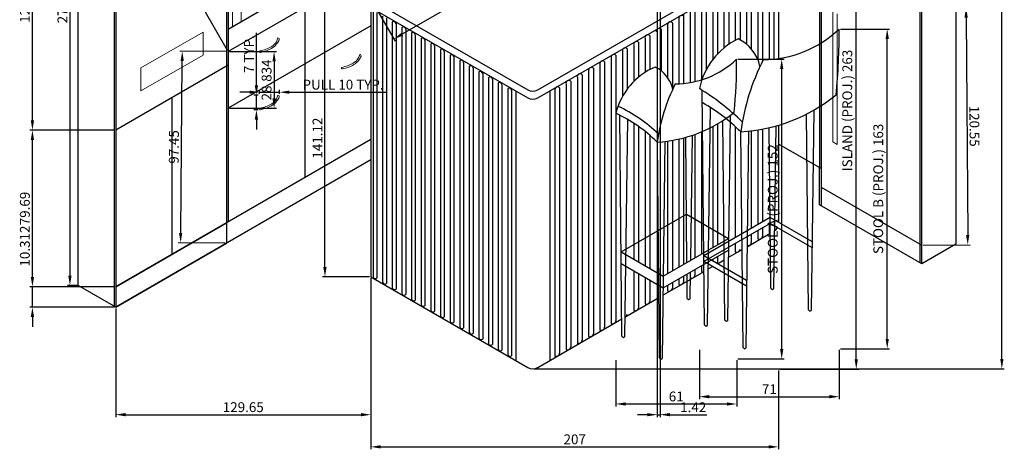
# Model space of a CAD drawing. Units: centimetres. Extents: x 2148 to 2649, y 4226 to 4785.
# Tile 1 of 6: x 2148 to 2649, y 4226 to 4445. Entities that reach past the tile are written whole.
import ezdxf

# ---------------------------------------------------------------- set-up
doc = ezdxf.new("R2010")
doc.units = ezdxf.units.CM
for name, color, linetype, lineweight in [('A-ANNO-DIMS', 63, 'Continuous', 18), ('A-ANNO-REFR', 8, 'Continuous', 13), ('A-EQPM', 30, 'Continuous', 18), ('A-FLOR-BSPL', 21, 'Continuous', 13), ('A-FLOR-CASE', 21, 'Continuous', 25), ('A-FLOR-CASE-HDW', 21, 'Continuous', 18), ('A-FLOR-CASE-TALL', 30, 'Continuous', 30), ('A-FLOR-CTOP', 21, 'Continuous', 25), ('CHAIR', 32, 'Continuous', 25), ('TABLE', 30, 'Continuous', 25)]:
    doc.layers.add(name, color=color, linetype=linetype, lineweight=lineweight)
doc.styles.get("Standard").update_dxf_attribs({"font": 'arial.ttf'})
doc.dimstyles.new('ISO-25', dxfattribs={"dimtxt": 5, "dimasz": 5, "dimexe": 1.25, "dimexo": 0.625, "dimtad": 1, "dimdec": 1, "dimtxsty": 'Standard', "dimcen": 2.5, "dimadec": 0, "dimazin": 0, "dimtfac": 1, "dimtdec": 1, "dimtmove": 0, "dimatfit": 3, "dimfxl": 1, "dimarcsym": 0})

# ---------------------------------------------------------------- blocks, each defined once
blk = doc.blocks.new('RECTANGLE')
for p, q in [((2256.66, 4502.65), (2260.99, 4505.15)), ((2260.99, 4443.76), (2260.99, 4505.15)), ((2256.66, 4502.65), (2256.66, 4441.26)), ((2256.66, 4441.26), (2260.99, 4443.76))]:
    blk.add_line(p, q)
blk = doc.blocks.new('*D4')
at = {"layer": 'A-ANNO-DIMS', "color": 0, "lineweight": -2, "transparency": 16777216}
for p, q in [((2177.63, 4587.69), (2172.75, 4587.69)), ((2174, 4582.69), (2174, 4314.69)), ((2177.63, 4309.69), (2172.75, 4309.69))]:
    blk.add_line(p, q, dxfattribs=at)
at = {"layer": 'A-ANNO-DIMS', "color": 0, "transparency": 16777216}
for points in [[(2173.16, 4582.69), (2174.83, 4582.69), (2174, 4587.69)], [(2173.16, 4314.69), (2174.83, 4314.69), (2174, 4309.69)]]:
    blk.add_solid(points, dxfattribs=at)
at = {"layer": 'Defpoints', "color": 0, "transparency": 16777216}
for p in [(2178.26, 4587.69), (2174, 4309.69), (2178.26, 4309.69)]:
    blk.add_point(p, dxfattribs=at)
at = {"layer": 'A-ANNO-DIMS', "color": 0, "transparency": 16777216, "insert": (2170.82, 4448.69), "char_height": 5, "attachment_point": 5, "rotation": 90}
blk.add_mtext('278', dxfattribs=at)
blk = doc.blocks.new('CHAIR')
for p, q in [((2681.59, 4311.07), (2681.04, 4368.06)), ((2683.02, 4367), (2682.28, 4310.87)), ((2708.11, 4315.21), (2707.62, 4366.68)), ((2709.5, 4367.99), (2708.8, 4315.01)), ((2691.26, 4305.48), (2690.73, 4361.11)), ((2692.69, 4361.28), (2691.95, 4305.29)), ((2698.34, 4330.07), (2698.03, 4362.34)), ((2699.68, 4362.84), (2699.25, 4330.6)), ((2681.38, 4332.81), (2698.22, 4342.54)), ((2698.22, 4342.54), (2709.08, 4336.27)), ((2692.23, 4326.55), (2709.08, 4336.27)), ((2692.23, 4323.55), (2709.08, 4333.27)), ((2681.38, 4332.81), (2692.23, 4326.55)), ((2681.38, 4329.81), (2692.23, 4323.55)), ((2698.43, 4320.79), (2698.37, 4327.09)), ((2699.21, 4327.58), (2699.12, 4320.6)), ((2698.43, 4320.79), (2698.84, 4320.47)), ((2698.84, 4320.47), (2699.12, 4320.6)), ((2708.11, 4315.21), (2708.52, 4314.89)), ((2708.52, 4314.89), (2708.8, 4315.01)), ((2681.59, 4311.07), (2682, 4310.75)), ((2682, 4310.75), (2682.28, 4310.87)), ((2691.26, 4305.48), (2691.67, 4305.16)), ((2691.67, 4305.16), (2691.95, 4305.29))]:
    blk.add_line(p, q)
for centre, radius, start, end in [((2695.17, 4399.34), 23.22, 270.4571, 313.5464), ((2570.59, 4382.17), 140.58, 354.5439, 0.1387), ((2697.23, 4364.18), 17.77, 113.5651, 165.7781), ((2686.69, 4373.07), 8.17, 11.759, 65.0744), ((2738.35, 4354.49), 48.13, 153.2927, 172.0917), ((2664.71, 4335.25), 36.64, 44.8785, 65.3279), ((2665.42, 4337.18), 36.47, 45.4434, 65.457), ((2688.67, 4395.75), 34.7, 273.3125, 309.0476)]:
    blk.add_arc(centre, radius, start, end)
blk = doc.blocks.new('CHAIR 2')
for p, q in [((2745.93, 4145.72), (2744.8, 4264.9)), ((2748.76, 4256.29), (2747.29, 4145.34)), ((2798.71, 4153.34), (2797.76, 4252.83)), ((2801.41, 4254.8), (2800.07, 4152.96)), ((2765.51, 4134.17), (2764.46, 4243.82)), ((2768.32, 4244.16), (2766.87, 4133.79)), ((2779.63, 4164.35), (2778.85, 4245.92)), ((2782.09, 4246.75), (2780.99, 4163.97)), ((2779.29, 4200.26), (2745.6, 4180.81)), ((2800.53, 4188), (2779.29, 4200.26)), ((2779.29, 4197.26), (2745.6, 4177.81)), ((2800.53, 4185), (2779.29, 4197.26)), ((2767.32, 4168.27), (2745.6, 4180.81)), ((2745.6, 4177.81), (2745.6, 4180.81)), ((2767.32, 4165.27), (2745.6, 4177.81)), ((2779.63, 4164.35), (2780.44, 4163.72)), ((2780.44, 4163.72), (2780.99, 4163.97)), ((2798.71, 4153.34), (2799.51, 4152.71)), ((2799.51, 4152.71), (2800.07, 4152.96)), ((2745.93, 4145.72), (2746.74, 4145.09)), ((2746.74, 4145.09), (2747.29, 4145.34)), ((2765.51, 4134.17), (2766.31, 4133.54)), ((2766.31, 4133.54), (2766.87, 4133.79))]:
    blk.add_line(p, q)
for centre, radius, start, end in [((2775.29, 4337.16), 56.71, 270.4571, 313.5464), ((2471.12, 4295.23), 343.24, 354.5439, 0.1387), ((2779.32, 4258.12), 36.79, 116.36, 167.9437), ((2754.58, 4273.01), 19.94, 11.759, 65.0744), ((2880.73, 4227.64), 117.53, 153.2927, 172.0917), ((2676.17, 4157.1), 127.79, 45.8786, 58.2873), ((2700.72, 4180.45), 89.78, 44.8855, 60.4426), ((2759.43, 4328.4), 84.73, 273.3125, 309.0476)]:
    blk.add_arc(centre, radius, start, end)
blk = doc.blocks.new('T')
for p, q in [((2448.14, 4353.09), (2318.24, 4278.09)), ((2522.91, 4309.92), (2448.14, 4353.09)), ((2403.01, 4232.03), (2522.91, 4301.26)), ((2318.24, 4278.09), (2398.01, 4232.03))]:
    blk.add_line(p, q)
for centre, start, end in [((2520.41, 4305.59), 300, 60), ((2400.51, 4236.36), 240, 300)]:
    blk.add_arc(centre, 5, start, end)
blk = doc.blocks.new('FRUITS')
for centre in [(2416.61, 4474.09), (2421.39, 4472.47), (2427.91, 4474), (2437.55, 4475.46)]:
    blk.add_circle(centre, 1.88)
for centre, start, end in [((2425.68, 4477.15), 250.6785, 228.1131), ((2431.37, 4476.49), 347.1742, 260.6235), ((2420.14, 4474.94), 339.5983, 177.9649), ((2420.14, 4474.94), 208.8656, 254.0869), ((2423.8, 4473.97), 252.9307, 170.9248), ((2432.9, 4474.21), 301.9934, 262.6603)]:
    blk.add_arc(centre, 1.88, start, end)
for start_param, end_param in [(4.471607, 4.914134), (5.976427, 9.8373)]:
    blk.add_ellipse((2418.08, 4470.84), major_axis=(-2.82, 1), ratio=0.809593, start_param=start_param, end_param=end_param)
for points, knots in [([(2406.43, 4471.88), (2412.49, 4474.08), (2424.62, 4478.48), (2437.33, 4476.24), (2443.7, 4475.12)], [0, 0, 0, 0, 18.967698, 37.99902, 37.99902, 37.99902, 37.99902]), ([(2406.43, 4471.88), (2409.22, 4465.94), (2414.78, 4454.12), (2438.7, 4455.69), (2442.02, 4468.59), (2443.7, 4475.12)], [0, 0, 0, 0, 18.249558, 36.298645, 54.808813, 54.808813, 54.808813, 54.808813]), ([(2406.43, 4471.88), (2411.36, 4471.29), (2423.93, 4469.77), (2436.23, 4473.1), (2443.7, 4475.12)], [0, 0, 0, 0, 14.783083, 37.710843, 37.710843, 37.710843, 37.710843])]:
    blk.add_open_spline(points, degree=3, knots=knots)
blk = doc.blocks.new('TABLE 3')
for p, q in [((2534.09, 4482.72), (2534.09, 4425.1)), ((2529.29, 4472.97), (2529.29, 4424.6)), ((2531.69, 4473.13), (2531.69, 4424.8)), ((2531.69, 4473.13), (2531.69, 4424.8)), ((2523.55, 4469.66), (2523.55, 4424.61)), ((2523.55, 4468.43), (2523.55, 4424.61)), ((2525.96, 4471.05), (2525.96, 4423.89)), ((2525.96, 4469.82), (2525.96, 4423.89)), ((2529.29, 4471.74), (2529.29, 4424.6)), ((2512.09, 4463.04), (2512.09, 4434.39)), ((2514.5, 4464.43), (2514.5, 4434.64)), ((2514.5, 4463.2), (2514.5, 4434.64)), ((2517.82, 4466.35), (2517.82, 4432.4)), ((2517.82, 4465.12), (2517.82, 4432.4)), ((2520.23, 4467.74), (2520.23, 4430.04)), ((2520.23, 4466.51), (2520.23, 4430.04)), ((2503.03, 4457.81), (2503.03, 4427.36)), ((2506.35, 4459.73), (2506.35, 4430.48)), ((2506.35, 4458.5), (2506.35, 4430.48)), ((2508.76, 4461.12), (2508.76, 4432.32)), ((2512.09, 4461.81), (2512.09, 4434.39)), ((2326.91, 4455.22), (2326.91, 4314.1)), ((2494.89, 4453.11), (2494.89, 4413.65)), ((2497.3, 4454.5), (2497.3, 4419.33)), ((2497.3, 4453.27), (2497.3, 4419.33)), ((2500.62, 4456.42), (2500.62, 4424.52)), ((2500.62, 4455.19), (2500.62, 4424.52)), ((2503.03, 4456.58), (2503.03, 4427.36)), ((2328.01, 4449.42), (2328.01, 4314.3)), ((2329.93, 4448.55), (2329.93, 4313.58)), ((2485.83, 4447.88), (2485.83, 4412.44)), ((2489.16, 4449.8), (2489.16, 4412.9)), ((2489.16, 4448.57), (2489.16, 4412.9)), ((2491.57, 4451.19), (2491.57, 4413.39)), ((2491.57, 4449.96), (2491.57, 4413.39)), ((2494.89, 4451.88), (2494.89, 4413.65)), ((2332.9, 4446.6), (2332.9, 4311.48)), ((2334.82, 4445.73), (2334.82, 4310.75)), ((2337.79, 4443.77), (2337.79, 4308.66)), ((2339.71, 4442.9), (2339.71, 4307.93)), ((2480.1, 4443.34), (2480.1, 4410.27)), ((2480.1, 4443.34), (2480.1, 4410.27)), ((2483.42, 4446.49), (2483.42, 4412.26)), ((2483.42, 4445.26), (2483.42, 4412.26)), ((2485.83, 4446.65), (2485.83, 4412.44)), ((2342.68, 4440.95), (2342.68, 4305.83)), ((2344.61, 4440.08), (2344.61, 4305.11)), ((2347.58, 4438.12), (2347.58, 4303.01)), ((2474.37, 4440.03), (2474.37, 4418.94)), ((2477.69, 4441.95), (2477.69, 4415.46)), ((2477.69, 4441.95), (2477.69, 4415.46)), ((2349.5, 4437.25), (2349.5, 4302.28)), ((2352.47, 4435.3), (2352.47, 4300.18)), ((2354.39, 4434.43), (2354.39, 4299.46)), ((2462.9, 4433.41), (2462.9, 4415.61)), ((2462.9, 4433.41), (2462.9, 4415.61)), ((2466.23, 4435.33), (2466.23, 4418.06)), ((2466.23, 4435.33), (2466.23, 4418.06)), ((2468.64, 4436.72), (2468.64, 4419.49)), ((2468.64, 4436.72), (2468.64, 4419.49)), ((2357.36, 4432.47), (2357.36, 4297.36)), ((2359.28, 4431.6), (2359.28, 4296.63)), ((2362.25, 4429.65), (2362.25, 4294.53)), ((2364.18, 4428.78), (2364.18, 4293.81)), ((2454.76, 4428.71), (2454.76, 4405.82)), ((2457.17, 4430.1), (2457.17, 4409.54)), ((2457.17, 4430.1), (2457.17, 4409.54)), ((2460.49, 4432.02), (2460.49, 4413.4)), ((2460.49, 4432.02), (2460.49, 4413.4)), ((2367.15, 4426.82), (2367.15, 4291.71)), ((2369.07, 4425.95), (2369.07, 4290.98)), ((2372.04, 4424), (2372.04, 4288.88)), ((2373.96, 4423.13), (2373.96, 4288.16)), ((2445.7, 4423.48), (2445.7, 4288.49)), ((2449.03, 4425.4), (2449.03, 4290.41)), ((2451.44, 4426.79), (2451.44, 4291.8)), ((2376.93, 4421.17), (2376.93, 4286.06)), ((2378.85, 4420.3), (2378.85, 4285.33)), ((2381.82, 4418.35), (2381.82, 4283.23)), ((2437.56, 4418.78), (2437.56, 4283.79)), ((2439.97, 4420.17), (2439.97, 4285.18)), ((2443.3, 4422.09), (2443.3, 4287.1)), ((2383.75, 4417.48), (2383.75, 4282.51)), ((2386.72, 4415.52), (2386.72, 4280.41)), ((2388.64, 4414.65), (2388.64, 4279.68)), ((2428.51, 4413.55), (2428.51, 4278.56)), ((2431.83, 4415.47), (2431.83, 4280.48)), ((2434.24, 4416.86), (2434.24, 4281.87)), ((2391.61, 4412.7), (2391.61, 4277.58)), ((2393.53, 4411.83), (2393.53, 4276.86)), ((2396.5, 4409.88), (2396.5, 4274.76)), ((2398.42, 4409.01), (2398.42, 4274.03)), ((2400.52, 4408.63), (2400.52, 4271.6)), ((2417.84, 4408.63), (2417.84, 4271.6)), ((2420.37, 4408.85), (2420.37, 4273.86)), ((2422.77, 4410.24), (2422.77, 4275.25)), ((2426.1, 4412.16), (2426.1, 4277.17)), ((2460.49, 4392.27), (2460.49, 4323.14)), ((2462.9, 4390.64), (2462.9, 4321.75)), ((2466.23, 4388.14), (2466.23, 4319.83)), ((2494.89, 4387.83), (2494.89, 4325.72)), ((2500.62, 4390.56), (2500.62, 4329.03)), ((2503.03, 4391.9), (2503.03, 4330.42)), ((2512.09, 4390.5), (2512.09, 4334.07)), ((2520.23, 4388.33), (2520.23, 4338.77)), ((2523.55, 4388.81), (2523.55, 4340.69)), ((2525.96, 4389.23), (2525.96, 4342.08)), ((2534.09, 4391.22), (2534.09, 4381.5)), ((2468.64, 4386.14), (2468.64, 4318.44)), ((2477.69, 4383.14), (2477.69, 4315.79)), ((2480.1, 4383.51), (2480.1, 4317.18)), ((2483.42, 4384.17), (2483.42, 4319.1)), ((2485.83, 4384.76), (2485.83, 4320.49)), ((2491.57, 4386.54), (2491.57, 4323.8)), ((2534.09, 4384.82), (2534.09, 4341.83)), ((2525.96, 4339.08), (2525.96, 4334.83)), ((2529.29, 4341), (2529.29, 4336.74)), ((2518.06, 4329.46), (2529.88, 4336.29)), ((2520.23, 4335.77), (2520.23, 4331.52)), ((2523.55, 4337.69), (2523.55, 4333.43)), ((2508.53, 4323.96), (2515.55, 4328.01)), ((2512.09, 4331.07), (2512.09, 4326.82)), ((2500.62, 4323.12), (2500.62, 4322.24)), ((2503.03, 4324.51), (2503.03, 4321.59)), ((2503.09, 4320.82), (2506.45, 4322.76)), ((2491.57, 4317.89), (2491.57, 4314.97)), ((2494.89, 4319.81), (2494.89, 4316.89)), ((2498.19, 4317.99), (2500.49, 4319.32)), ((2326.91, 4314.1), (2406.68, 4268.04)), ((2460.49, 4317.23), (2460.49, 4297.03)), ((2462.9, 4315.84), (2462.9, 4298.42)), ((2466.23, 4313.92), (2466.23, 4300.34)), ((2475.33, 4304.79), (2496.19, 4316.83)), ((2483.42, 4313.19), (2483.42, 4310.27)), ((2485.83, 4314.58), (2485.83, 4311.66)), ((2489.16, 4316.5), (2489.16, 4313.58)), ((2468.64, 4312.53), (2468.64, 4301.73)), ((2477.69, 4309.88), (2477.69, 4306.96)), ((2480.1, 4311.27), (2480.1, 4308.35)), ((2455.96, 4293.61), (2473.25, 4303.59)), ((2411.68, 4268.04), (2454.39, 4292.7))]:
    blk.add_line(p, q)
for centre, radius, start, end in [((2530.67, 4472.12), 1.44, 44.5272, 195.4728), ((2524.94, 4468.81), 1.44, 44.5272, 195.4728), ((2513.47, 4462.19), 1.44, 44.5272, 195.4728), ((2519.2, 4465.5), 1.44, 44.5272, 195.4728), ((2507.74, 4458.88), 1.44, 44.5272, 195.4728), ((2496.27, 4452.26), 1.44, 44.5272, 195.4728), ((2502.01, 4455.57), 1.44, 44.5272, 195.4728), ((2490.54, 4448.95), 1.44, 44.5272, 195.4728), ((2479.08, 4442.33), 1.44, 44.5272, 195.4728), ((2484.81, 4445.64), 1.44, 44.5272, 195.4728), ((2473.34, 4439.02), 1.44, 44.5272, 195.4728), ((2461.88, 4432.4), 1.44, 44.5272, 195.4728), ((2467.61, 4435.71), 1.44, 44.5272, 195.4728), ((2456.15, 4429.09), 1.44, 44.5272, 195.4728), ((2444.68, 4422.47), 1.44, 44.5272, 195.4728), ((2450.41, 4425.78), 1.44, 44.5272, 195.4728), ((2438.95, 4419.16), 1.44, 44.5272, 195.4728), ((2427.48, 4412.55), 1.44, 44.5272, 195.4728), ((2433.22, 4415.85), 1.44, 44.5272, 195.4728), ((2421.75, 4409.24), 1.44, 44.5272, 195.4728), ((2529.09, 4341.6), 5, 304.2234, 331.1295), ((2524.24, 4335.03), 1.74, 246.8122, 353.1878), ((2529.97, 4338.34), 1.74, 246.8122, 267.0744), ((2512.77, 4328.41), 1.74, 246.8122, 353.1878), ((2518.5, 4331.72), 1.74, 255.6127, 353.1878), ((2501.31, 4321.79), 1.74, 331.6217, 353.1878), ((2329.13, 4314.36), 1.12, 182.9367, 315.698), ((2489.84, 4315.17), 1.74, 246.8122, 353.1878), ((2495.57, 4318.48), 1.74, 246.8122, 290.8785), ((2334.02, 4311.54), 1.12, 182.9367, 315.698), ((2338.91, 4308.71), 1.12, 182.9367, 315.698), ((2478.38, 4308.55), 1.74, 246.8122, 353.1878), ((2484.11, 4311.86), 1.74, 246.8122, 353.1878), ((2343.8, 4305.89), 1.12, 182.9367, 315.698), ((2348.7, 4303.06), 1.12, 182.9367, 315.698), ((2353.59, 4300.24), 1.12, 182.9367, 315.698), ((2461.18, 4298.62), 1.74, 246.8122, 353.1878), ((2466.91, 4301.93), 1.74, 246.8122, 353.1878), ((2358.48, 4297.41), 1.12, 182.9367, 315.698), ((2363.37, 4294.59), 1.12, 182.9367, 315.698), ((2455.45, 4295.31), 1.74, 287.3713, 353.1878), ((2368.27, 4291.77), 1.12, 182.9367, 315.698), ((2373.16, 4288.94), 1.12, 182.9367, 315.698), ((2443.98, 4288.7), 1.74, 246.8122, 353.1878), ((2449.71, 4292.01), 1.74, 246.8122, 353.1878), ((2378.05, 4286.12), 1.12, 182.9367, 315.698), ((2382.94, 4283.29), 1.12, 182.9367, 315.698), ((2438.25, 4285.39), 1.74, 246.8122, 353.1878), ((2387.84, 4280.47), 1.12, 182.9367, 315.698), ((2426.78, 4278.77), 1.74, 246.8122, 353.1878), ((2432.51, 4282.08), 1.74, 246.8122, 353.1878), ((2392.73, 4277.64), 1.12, 182.9367, 315.698), ((2397.62, 4274.82), 1.12, 182.9367, 315.698), ((2421.05, 4275.46), 1.74, 246.8122, 353.1878), ((2409.18, 4272.37), 5, 240, 300)]:
    blk.add_arc(centre, radius, start, end)
for name, p in [('T', (8.67, 177.13)), ('T', (8.67, 173.04)), ('FRUITS', (0, 0))]:
    blk.add_blockref(name, p)
blk = doc.blocks.new('PULL-BASE-BOW')
for centre, radius, start, end in [((9.29, 6.64), 0.774, 341.702, 83.222), ((0.41, 0.41), 0.414, 116.0189, 282.6641)]:
    blk.add_arc(centre, radius, start, end)
for points, knots in [([(0.23, 0.79), (2.23, 1.29), (5.42, 2.1), (8.53, 4.9), (9.15, 6.73), (9.38, 7.41)], [0, 0, 0, 0, 6.127515, 9.756066, 11.887711, 11.887711, 11.887711, 11.887711]), ([(0.5, 0.01), (2.55, 0.54), (5.72, 1.35), (8.78, 4.08), (9.68, 5.75), (10.03, 6.4)], [0, 0, 0, 0, 6.234589, 9.67204, 11.894402, 11.894402, 11.894402, 11.894402])]:
    blk.add_open_spline(points, degree=3, knots=knots)
blk = doc.blocks.new('*D22')
at = {"layer": 'A-ANNO-DIMS', "color": 0, "lineweight": -2, "transparency": 16777216}
for p, q in [((2265.28, 4408.01), (2260.28, 4408.01)), ((2270.28, 4407.11), (2270.28, 4409.26)), ((2270.28, 4408.01), (2280.42, 4408.01)), ((2280.42, 4407.11), (2280.42, 4409.26)), ((2285.42, 4408.01), (2335.17, 4408.01))]:
    blk.add_line(p, q, dxfattribs=at)
at = {"layer": 'A-ANNO-DIMS', "color": 0, "transparency": 16777216}
for points in [[(2265.28, 4408.84), (2265.28, 4407.18), (2270.28, 4408.01)], [(2285.42, 4408.84), (2285.42, 4407.18), (2280.42, 4408.01)]]:
    blk.add_solid(points, dxfattribs=at)
at = {"layer": 'Defpoints', "color": 0, "transparency": 16777216}
for p in [(2280.42, 4408.01), (2270.28, 4406.49), (2280.42, 4406.49)]:
    blk.add_point(p, dxfattribs=at)
at = {"layer": 'A-ANNO-DIMS', "color": 0, "transparency": 16777216, "insert": (2312.8, 4411.19), "char_height": 5, "attachment_point": 5}
blk.add_mtext('PULL 10 TYP.', dxfattribs=at)
blk = doc.blocks.new('*D23')
at = {"layer": 'A-ANNO-DIMS', "color": 0, "lineweight": -2, "transparency": 16777216}
for p, q in [((2268.75, 4411.49), (2268.75, 4438.15)), ((2269.65, 4406.49), (2267.5, 4406.49)), ((2268.75, 4399.04), (2268.75, 4406.49)), ((2269.65, 4399.04), (2267.5, 4399.04)), ((2268.75, 4394.04), (2268.75, 4389.04))]:
    blk.add_line(p, q, dxfattribs=at)
at = {"layer": 'A-ANNO-DIMS', "color": 0, "transparency": 16777216}
for points in [[(2267.92, 4411.49), (2269.59, 4411.49), (2268.75, 4406.49)], [(2267.92, 4394.04), (2269.59, 4394.04), (2268.75, 4399.04)]]:
    blk.add_solid(points, dxfattribs=at)
at = {"layer": 'Defpoints', "color": 0, "transparency": 16777216}
for p in [(2268.75, 4406.49), (2270.28, 4406.49), (2270.28, 4399.04)]:
    blk.add_point(p, dxfattribs=at)
at = {"layer": 'A-ANNO-DIMS', "color": 0, "transparency": 16777216, "insert": (2265.63, 4427.32), "char_height": 5, "attachment_point": 5, "rotation": 90}
blk.add_mtext('7 TYP.', dxfattribs=at)
blk = doc.blocks.new('*D30')
at = {"layer": 'A-ANNO-DIMS', "color": 0, "lineweight": -2, "transparency": 16777216}
for p, q in [((2534.71, 4530.22), (2574.8, 4530.22)), ((2573.55, 4272.15), (2573.55, 4525.22)), ((2534.71, 4267.15), (2574.8, 4267.15))]:
    blk.add_line(p, q, dxfattribs=at)
at = {"layer": 'A-ANNO-DIMS', "color": 0, "transparency": 16777216}
for points in [[(2572.71, 4525.22), (2574.38, 4525.22), (2573.55, 4530.22)], [(2572.71, 4272.15), (2574.38, 4272.15), (2573.55, 4267.15)]]:
    blk.add_solid(points, dxfattribs=at)
at = {"layer": 'Defpoints', "color": 0, "transparency": 16777216}
for p in [(2534.09, 4530.22), (2573.55, 4530.22), (2534.09, 4267.15)]:
    blk.add_point(p, dxfattribs=at)
at = {"layer": 'A-ANNO-DIMS', "color": 0, "transparency": 16777216, "insert": (2569.64, 4398.69), "char_height": 5, "attachment_point": 5, "rotation": 90}
blk.add_mtext('ISLAND (PROJ.) 263', dxfattribs=at)
blk = doc.blocks.new('*D31')
at = {"layer": 'A-ANNO-DIMS', "color": 0, "lineweight": -2, "transparency": 16777216}
for p, q in [((2326.91, 4266.52), (2326.91, 4226.44)), ((2534.09, 4266.52), (2534.09, 4226.44)), ((2331.91, 4227.69), (2529.09, 4227.69))]:
    blk.add_line(p, q, dxfattribs=at)
at = {"layer": 'A-ANNO-DIMS', "color": 0, "transparency": 16777216}
for points in [[(2331.91, 4228.52), (2331.91, 4226.86), (2326.91, 4227.69)], [(2529.09, 4228.52), (2529.09, 4226.86), (2534.09, 4227.69)]]:
    blk.add_solid(points, dxfattribs=at)
at = {"layer": 'Defpoints', "color": 0, "transparency": 16777216}
for p in [(2326.91, 4267.15), (2534.09, 4267.15), (2534.09, 4227.69)]:
    blk.add_point(p, dxfattribs=at)
at = {"layer": 'A-ANNO-DIMS', "color": 0, "transparency": 16777216, "insert": (2430.5, 4230.87), "char_height": 5, "attachment_point": 5}
blk.add_mtext('207', dxfattribs=at)
blk = doc.blocks.new('*D32')
at = {"layer": 'A-ANNO-DIMS', "color": 0, "lineweight": -2, "transparency": 16777216}
for p, q in [((2513.43, 4424.81), (2536.92, 4424.81)), ((2535.67, 4277.36), (2535.67, 4419.81)), ((2513.43, 4272.36), (2536.92, 4272.36))]:
    blk.add_line(p, q, dxfattribs=at)
at = {"layer": 'A-ANNO-DIMS', "color": 0, "transparency": 16777216}
for points in [[(2534.84, 4419.81), (2536.5, 4419.81), (2535.67, 4424.81)], [(2534.84, 4277.36), (2536.5, 4277.36), (2535.67, 4272.36)]]:
    blk.add_solid(points, dxfattribs=at)
at = {"layer": 'Defpoints', "color": 0, "transparency": 16777216}
for p in [(2512.8, 4424.81), (2535.67, 4424.81), (2512.8, 4272.36)]:
    blk.add_point(p, dxfattribs=at)
at = {"layer": 'A-ANNO-DIMS', "color": 0, "transparency": 16777216, "insert": (2531.77, 4348.58), "char_height": 5, "attachment_point": 5, "rotation": 90}
blk.add_mtext('STOOL A (PROJ.) 152', dxfattribs=at)
blk = doc.blocks.new('*D33')
at = {"layer": 'A-ANNO-DIMS', "color": 0, "lineweight": -2, "transparency": 16777216}
for p, q in [((2451.36, 4271.73), (2451.36, 4248.24)), ((2512.8, 4271.73), (2512.8, 4248.24)), ((2456.36, 4249.49), (2507.8, 4249.49))]:
    blk.add_line(p, q, dxfattribs=at)
at = {"layer": 'A-ANNO-DIMS', "color": 0, "transparency": 16777216}
for points in [[(2456.36, 4250.32), (2456.36, 4248.65), (2451.36, 4249.49)], [(2507.8, 4250.32), (2507.8, 4248.65), (2512.8, 4249.49)]]:
    blk.add_solid(points, dxfattribs=at)
at = {"layer": 'Defpoints', "color": 0, "transparency": 16777216}
for p in [(2451.36, 4272.36), (2512.8, 4272.36), (2512.8, 4249.49)]:
    blk.add_point(p, dxfattribs=at)
at = {"layer": 'A-ANNO-DIMS', "color": 0, "transparency": 16777216, "insert": (2482.08, 4252.67), "char_height": 5, "attachment_point": 5}
blk.add_mtext('61', dxfattribs=at)
blk = doc.blocks.new('*D34')
at = {"layer": 'A-ANNO-DIMS', "color": 0, "lineweight": -2, "transparency": 16777216}
for p, q in [((2565.53, 4440.1), (2590.53, 4440.1)), ((2589.28, 4282.58), (2589.28, 4435.1)), ((2565.53, 4277.58), (2590.53, 4277.58))]:
    blk.add_line(p, q, dxfattribs=at)
at = {"layer": 'A-ANNO-DIMS', "color": 0, "transparency": 16777216}
for points in [[(2588.45, 4435.1), (2590.12, 4435.1), (2589.28, 4440.1)], [(2588.45, 4282.58), (2590.12, 4282.58), (2589.28, 4277.58)]]:
    blk.add_solid(points, dxfattribs=at)
at = {"layer": 'Defpoints', "color": 0, "transparency": 16777216}
for p in [(2564.9, 4440.1), (2589.28, 4440.1), (2564.9, 4277.58)]:
    blk.add_point(p, dxfattribs=at)
at = {"layer": 'A-ANNO-DIMS', "color": 0, "transparency": 16777216, "insert": (2585.38, 4358.84), "char_height": 5, "attachment_point": 5, "rotation": 90}
blk.add_mtext('STOOL B (PROJ.) 163', dxfattribs=at)
blk = doc.blocks.new('*D35')
at = {"layer": 'A-ANNO-DIMS', "color": 0, "lineweight": -2, "transparency": 16777216}
for p, q in [((2493.86, 4276.95), (2493.86, 4251.95)), ((2564.9, 4276.95), (2564.9, 4251.95)), ((2498.86, 4253.2), (2559.9, 4253.2))]:
    blk.add_line(p, q, dxfattribs=at)
at = {"layer": 'A-ANNO-DIMS', "color": 0, "transparency": 16777216}
for points in [[(2498.86, 4254.04), (2498.86, 4252.37), (2493.86, 4253.2)], [(2559.9, 4254.04), (2559.9, 4252.37), (2564.9, 4253.2)]]:
    blk.add_solid(points, dxfattribs=at)
at = {"layer": 'Defpoints', "color": 0, "transparency": 16777216}
for p in [(2493.86, 4277.58), (2564.9, 4277.58), (2564.9, 4253.2)]:
    blk.add_point(p, dxfattribs=at)
at = {"layer": 'A-ANNO-DIMS', "color": 0, "transparency": 16777216, "insert": (2529.38, 4256.34), "char_height": 5, "attachment_point": 5}
blk.add_mtext('71', dxfattribs=at)
blk = doc.blocks.new('*D48')
at = {"layer": 'A-ANNO-DIMS', "color": 0, "lineweight": -2, "transparency": 16777216}
for p, q in [((2472.44, 4594.86), (2472.44, 4242.8)), ((2473.86, 4594.94), (2473.86, 4242.8)), ((2467.44, 4244.05), (2462.44, 4244.05)), ((2472.44, 4244.05), (2473.86, 4244.05)), ((2478.86, 4244.05), (2497.57, 4244.05))]:
    blk.add_line(p, q, dxfattribs=at)
at = {"layer": 'A-ANNO-DIMS', "color": 0, "transparency": 16777216}
for points in [[(2467.44, 4244.88), (2467.44, 4243.21), (2472.44, 4244.05)], [(2478.86, 4244.88), (2478.86, 4243.21), (2473.86, 4244.05)]]:
    blk.add_solid(points, dxfattribs=at)
at = {"layer": 'Defpoints', "color": 0, "transparency": 16777216}
for p in [(2472.44, 4595.48), (2473.86, 4595.56), (2473.86, 4244.05)]:
    blk.add_point(p, dxfattribs=at)
at = {"layer": 'A-ANNO-DIMS', "color": 0, "transparency": 16777216, "insert": (2490.71, 4247.18), "char_height": 5, "attachment_point": 5}
blk.add_mtext('1.42', dxfattribs=at)
blk = doc.blocks.new('*D51')
at = {"layer": 'A-ANNO-DIMS', "color": 0, "lineweight": -2, "transparency": 16777216}
for p, q in [((2436.91, 4714.24), (2648.78, 4714.24)), ((2647.53, 4272.37), (2647.53, 4709.24)), ((2409.81, 4267.37), (2648.78, 4267.37))]:
    blk.add_line(p, q, dxfattribs=at)
at = {"layer": 'A-ANNO-DIMS', "color": 0, "transparency": 16777216}
for points in [[(2646.7, 4709.24), (2648.37, 4709.24), (2647.53, 4714.24)], [(2646.7, 4272.37), (2648.37, 4272.37), (2647.53, 4267.37)]]:
    blk.add_solid(points, dxfattribs=at)
at = {"layer": 'Defpoints', "color": 0, "transparency": 16777216}
for p in [(2436.28, 4714.24), (2647.53, 4714.24), (2409.18, 4267.37)]:
    blk.add_point(p, dxfattribs=at)
at = {"layer": 'A-ANNO-DIMS', "color": 0, "transparency": 16777216, "insert": (2644.36, 4490.81), "char_height": 5, "attachment_point": 5, "rotation": 90}
blk.add_mtext('446.9', dxfattribs=at)
blk = doc.blocks.new('*D52')
at = {"layer": 'A-ANNO-DIMS', "color": 0, "lineweight": -2, "transparency": 16777216}
for p, q in [((2154.93, 4314.03), (2154.93, 4340.51)), ((2196.63, 4309.03), (2153.68, 4309.03)), ((2154.93, 4298.72), (2154.93, 4309.03)), ((2196.63, 4298.72), (2153.68, 4298.72)), ((2154.93, 4293.72), (2154.93, 4288.72))]:
    blk.add_line(p, q, dxfattribs=at)
at = {"layer": 'A-ANNO-DIMS', "color": 0, "transparency": 16777216}
for points in [[(2154.1, 4314.03), (2155.77, 4314.03), (2154.93, 4309.03)], [(2154.1, 4293.72), (2155.77, 4293.72), (2154.93, 4298.72)]]:
    blk.add_solid(points, dxfattribs=at)
at = {"layer": 'Defpoints', "color": 0, "transparency": 16777216}
for p in [(2154.93, 4309.03), (2197.26, 4309.03), (2197.26, 4298.72)]:
    blk.add_point(p, dxfattribs=at)
at = {"layer": 'A-ANNO-DIMS', "color": 0, "transparency": 16777216, "insert": (2151.75, 4329.77), "char_height": 5, "attachment_point": 5, "rotation": 90}
blk.add_mtext('10.312', dxfattribs=at)
blk = doc.blocks.new('*D53')
at = {"layer": 'A-ANNO-DIMS', "color": 0, "lineweight": -2, "transparency": 16777216}
for p, q in [((2196.63, 4388.72), (2153.68, 4388.72)), ((2154.93, 4314.03), (2154.93, 4383.72)), ((2196.63, 4309.03), (2153.68, 4309.03))]:
    blk.add_line(p, q, dxfattribs=at)
at = {"layer": 'A-ANNO-DIMS', "color": 0, "transparency": 16777216}
for points in [[(2154.1, 4383.72), (2155.77, 4383.72), (2154.93, 4388.72)], [(2154.1, 4314.03), (2155.77, 4314.03), (2154.93, 4309.03)]]:
    blk.add_solid(points, dxfattribs=at)
at = {"layer": 'Defpoints', "color": 0, "transparency": 16777216}
for p in [(2154.93, 4388.72), (2197.26, 4388.72), (2197.26, 4309.03)]:
    blk.add_point(p, dxfattribs=at)
at = {"layer": 'A-ANNO-DIMS', "color": 0, "transparency": 16777216, "insert": (2151.75, 4348.87), "char_height": 5, "attachment_point": 5, "rotation": 90}
blk.add_mtext('79.69', dxfattribs=at)
blk = doc.blocks.new('*D54')
at = {"layer": 'A-ANNO-DIMS', "color": 0, "lineweight": -2, "transparency": 16777216}
for p, q in [((2196.63, 4518.66), (2153.68, 4518.66)), ((2154.93, 4393.72), (2154.93, 4513.66)), ((2196.63, 4388.72), (2153.68, 4388.72))]:
    blk.add_line(p, q, dxfattribs=at)
at = {"layer": 'A-ANNO-DIMS', "color": 0, "transparency": 16777216}
for points in [[(2154.1, 4513.66), (2155.77, 4513.66), (2154.93, 4518.66)], [(2154.1, 4393.72), (2155.77, 4393.72), (2154.93, 4388.72)]]:
    blk.add_solid(points, dxfattribs=at)
at = {"layer": 'Defpoints', "color": 0, "transparency": 16777216}
for p in [(2154.93, 4518.66), (2197.26, 4518.66), (2197.26, 4388.72)]:
    blk.add_point(p, dxfattribs=at)
at = {"layer": 'A-ANNO-DIMS', "color": 0, "transparency": 16777216, "insert": (2151.75, 4453.69), "char_height": 5, "attachment_point": 5, "rotation": 90}
blk.add_mtext('129.94', dxfattribs=at)
blk = doc.blocks.new('*D55')
at = {"layer": 'A-ANNO-DIMS', "color": 0, "lineweight": -2, "transparency": 16777216}
for p, q in [((2253.79, 4428.66), (2229.84, 4428.88)), ((2230.27, 4336.42), (2231.05, 4423.86)), ((2252.92, 4331.22), (2228.98, 4331.43))]:
    blk.add_line(p, q, dxfattribs=at)
at = {"layer": 'A-ANNO-DIMS', "color": 0, "transparency": 16777216}
for points in [[(2230.21, 4423.87), (2231.88, 4423.86), (2231.09, 4428.86)], [(2229.44, 4336.43), (2231.1, 4336.41), (2230.23, 4331.42)]]:
    blk.add_solid(points, dxfattribs=at)
at = {"layer": 'Defpoints', "color": 0, "transparency": 16777216}
for p in [(2231.09, 4428.86), (2254.42, 4428.66), (2253.55, 4331.22)]:
    blk.add_point(p, dxfattribs=at)
at = {"layer": 'A-ANNO-DIMS', "color": 0, "transparency": 16777216, "insert": (2227.48, 4380.17), "char_height": 5, "attachment_point": 5, "rotation": 89.4908}
blk.add_mtext('97.45', dxfattribs=at)
blk = doc.blocks.new('*D56')
at = {"layer": 'A-ANNO-DIMS', "color": 0, "lineweight": -2, "transparency": 16777216}
for p, q in [((2326.29, 4455.22), (2302.34, 4455.22)), ((2303.59, 4319.1), (2303.59, 4450.22)), ((2326.29, 4314.1), (2302.34, 4314.1))]:
    blk.add_line(p, q, dxfattribs=at)
at = {"layer": 'A-ANNO-DIMS', "color": 0, "transparency": 16777216}
for points in [[(2302.75, 4450.22), (2304.42, 4450.22), (2303.59, 4455.22)], [(2302.75, 4319.1), (2304.42, 4319.1), (2303.59, 4314.1)]]:
    blk.add_solid(points, dxfattribs=at)
at = {"layer": 'Defpoints', "color": 0, "transparency": 16777216}
for p in [(2303.59, 4455.22), (2326.91, 4455.22), (2326.91, 4314.1)]:
    blk.add_point(p, dxfattribs=at)
at = {"layer": 'A-ANNO-DIMS', "color": 0, "transparency": 16777216, "insert": (2300.45, 4384.66), "char_height": 5, "attachment_point": 5, "rotation": 90}
blk.add_mtext('141.12', dxfattribs=at)
blk = doc.blocks.new('*D57')
at = {"layer": 'A-ANNO-DIMS', "color": 0, "lineweight": -2, "transparency": 16777216}
for p, q in [((2326.91, 4313.47), (2326.91, 4242.8)), ((2197.26, 4298.09), (2197.26, 4242.8)), ((2202.26, 4244.05), (2321.91, 4244.05))]:
    blk.add_line(p, q, dxfattribs=at)
at = {"layer": 'A-ANNO-DIMS', "color": 0, "transparency": 16777216}
for points in [[(2202.26, 4244.88), (2202.26, 4243.21), (2197.26, 4244.05)], [(2321.91, 4244.88), (2321.91, 4243.21), (2326.91, 4244.05)]]:
    blk.add_solid(points, dxfattribs=at)
at = {"layer": 'Defpoints', "color": 0, "transparency": 16777216}
for p in [(2326.91, 4314.1), (2197.26, 4298.72), (2326.91, 4244.05)]:
    blk.add_point(p, dxfattribs=at)
at = {"layer": 'A-ANNO-DIMS', "color": 0, "transparency": 16777216, "insert": (2262.08, 4247.23), "char_height": 5, "attachment_point": 5}
blk.add_mtext('129.65', dxfattribs=at)
blk = doc.blocks.new('*D58')
at = {"layer": 'A-ANNO-DIMS', "color": 0, "lineweight": -2, "transparency": 16777216}
for p, q in [((2457.13, 4529.68), (2469.1, 4508.94)), ((2464.15, 4507.52), (2342.9, 4437.52)), ((2327.22, 4454.68), (2339.2, 4433.94))]:
    blk.add_line(p, q, dxfattribs=at)
at = {"layer": 'A-ANNO-DIMS', "color": 0, "transparency": 16777216}
for points in [[(2463.73, 4508.25), (2464.56, 4506.8), (2468.48, 4510.02)], [(2342.49, 4438.25), (2343.32, 4436.8), (2338.57, 4435.02)]]:
    blk.add_solid(points, dxfattribs=at)
at = {"layer": 'Defpoints', "color": 0, "transparency": 16777216}
for p in [(2456.81, 4530.22), (2326.91, 4455.22), (2338.57, 4435.02)]:
    blk.add_point(p, dxfattribs=at)
at = {"layer": 'A-ANNO-DIMS', "color": 0, "transparency": 16777216, "insert": (2401.94, 4475.28), "char_height": 5, "attachment_point": 5, "rotation": 30}
blk.add_mtext('150', dxfattribs=at)
blk = doc.blocks.new('*D65')
at = {"layer": 'A-ANNO-DIMS', "color": 0, "lineweight": -2, "transparency": 16777216}
for p, q in [((2606.65, 4450.81), (2630.6, 4450.98)), ((2629.38, 4445.97), (2630.18, 4335.42)), ((2607.51, 4330.26), (2631.46, 4330.43))]:
    blk.add_line(p, q, dxfattribs=at)
at = {"layer": 'A-ANNO-DIMS', "color": 0, "transparency": 16777216}
for points in [[(2630.22, 4445.98), (2628.55, 4445.97), (2629.35, 4450.97)], [(2631.01, 4335.43), (2629.34, 4335.42), (2630.21, 4330.42)]]:
    blk.add_solid(points, dxfattribs=at)
at = {"layer": 'Defpoints', "color": 0, "transparency": 16777216}
for p in [(2606.02, 4450.81), (2606.89, 4330.26), (2630.21, 4330.42)]:
    blk.add_point(p, dxfattribs=at)
at = {"layer": 'A-ANNO-DIMS', "color": 0, "transparency": 16777216, "insert": (2632.96, 4390.72), "char_height": 5, "attachment_point": 5, "rotation": 270.4116}
blk.add_mtext('120.55', dxfattribs=at)
blk = doc.blocks.new('*D66')
at = {"layer": 'A-ANNO-DIMS', "color": 0, "lineweight": -2, "transparency": 16777216}
for p, q in [((2247.08, 4451.36), (2277.39, 4468.86)), ((2293.07, 4451.7), (2281.1, 4472.44)), ((2254.1, 4429.2), (2242.13, 4449.94))]:
    blk.add_line(p, q, dxfattribs=at)
at = {"layer": 'A-ANNO-DIMS', "color": 0, "transparency": 16777216}
for points in [[(2276.98, 4469.58), (2277.81, 4468.14), (2281.72, 4471.36)], [(2246.67, 4452.08), (2247.5, 4450.64), (2242.75, 4448.86)]]:
    blk.add_solid(points, dxfattribs=at)
at = {"layer": 'Defpoints', "color": 0, "transparency": 16777216}
for p in [(2281.72, 4471.36), (2293.39, 4451.16), (2254.42, 4428.66)]:
    blk.add_point(p, dxfattribs=at)
at = {"layer": 'A-ANNO-DIMS', "color": 0, "transparency": 16777216, "insert": (2260.66, 4462.85), "char_height": 5, "attachment_point": 5, "rotation": 30}
blk.add_mtext('45', dxfattribs=at)
blk = doc.blocks.new('*D67')
at = {"layer": 'A-ANNO-DIMS', "color": 0, "lineweight": -2, "transparency": 16777216}
for p, q in [((2255.04, 4428.66), (2278.99, 4428.66)), ((2277.74, 4423.66), (2277.74, 4404.82)), ((2255.04, 4399.82), (2278.99, 4399.82))]:
    blk.add_line(p, q, dxfattribs=at)
at = {"layer": 'A-ANNO-DIMS', "color": 0, "transparency": 16777216}
for points in [[(2276.91, 4423.66), (2278.57, 4423.66), (2277.74, 4428.66)], [(2276.91, 4404.82), (2278.57, 4404.82), (2277.74, 4399.82)]]:
    blk.add_solid(points, dxfattribs=at)
at = {"layer": 'Defpoints', "color": 0, "transparency": 16777216}
for p in [(2254.42, 4428.66), (2254.42, 4399.82), (2277.74, 4399.82)]:
    blk.add_point(p, dxfattribs=at)
at = {"layer": 'A-ANNO-DIMS', "color": 0, "transparency": 16777216, "insert": (2274.56, 4414.24), "char_height": 5, "attachment_point": 5, "rotation": 90}
blk.add_mtext('28.834', dxfattribs=at)

msp = doc.modelspace()

# ---------------------------------------------------------------- linework, layer by layer
at = {"layer": 'A-ANNO-REFR'}
msp.add_point((2293.387, 4422.323), dxfattribs=at)
at = {"layer": 'A-EQPM'}
for p, q in [((2197.2581, 4513.2764), (2197.2581, 4388.7152)), ((2210.001, 4420.322), (2241.673, 4438.6079)), ((2241.673, 4438.6079), (2241.673, 4426.9026)), ((2241.673, 4426.9026), (2210.001, 4408.6168)), ((2210.001, 4408.6168), (2210.001, 4420.322))]:
    msp.add_line(p, q, dxfattribs=at)
at = {"layer": 'A-FLOR-CASE'}
for p, q in [((2254.4158, 4609.2447), (2254.4158, 4342.0267)), ((2293.387, 4451.1569), (2293.387, 4364.5267)), ((2326.9105, 4441.6779), (2254.4158, 4399.823)), ((2326.9105, 4383.8816), (2197.2581, 4309.0267)), ((2555.7927, 4369.2793), (2534.0868, 4381.505)), ((2326.9105, 4373.57), (2197.2581, 4298.7152))]:
    msp.add_line(p, q, dxfattribs=at)
at = {"layer": 'A-FLOR-CASE-HDW'}
for p, q in [((2561.585, 4450.2388), (2561.585, 4382.7199)), ((2563.8432, 4381.4161), (2563.8432, 4447.8355)), ((2561.585, 4382.7199), (2563.8432, 4381.4161))]:
    msp.add_line(p, q, dxfattribs=at)
at = {"layer": 'A-FLOR-CASE-TALL'}
for p, q in [((2554.9266, 4645.7447), (2554.9266, 4369.7671)), ((2253.5498, 4608.7447), (2253.5498, 4331.2152)), ((2624.2087, 4605.7447), (2624.2087, 4330.7447)), ((2606.8882, 4320.7447), (2606.8882, 4595.7447)), ((2178.2568, 4309.6856), (2178.2568, 4587.6856)), ((2196.3921, 4577.2152), (2196.3921, 4299.2152)), ((2197.2581, 4576.2447), (2197.2581, 4298.7152)), ((2555.7927, 4561.7324), (2555.7927, 4350.2447)), ((2606.0221, 4321.2447), (2606.0221, 4532.7324)), ((2254.4158, 4421.7152), (2197.2581, 4388.7152)), ((2225.837, 4405.2152), (2225.837, 4325.5267)), ((2554.9266, 4350.7447), (2554.9266, 4369.7671)), ((2555.7927, 4359.7559), (2606.8882, 4330.2559)), ((2606.8882, 4320.7447), (2554.9266, 4350.7447)), ((2197.2581, 4309.0267), (2253.5498, 4341.5267)), ((2197.2581, 4298.7152), (2253.5498, 4331.2152)), ((2624.2087, 4330.7447), (2606.8882, 4320.7447)), ((2197.2581, 4298.7152), (2178.2568, 4309.6856))]:
    msp.add_line(p, q, dxfattribs=at)
at = {"layer": 'A-FLOR-CTOP'}
for p, q in [((2410.3004, 4529.9623), (2254.4158, 4439.9623)), ((2410.3004, 4518.6569), (2254.4158, 4428.6569))]:
    msp.add_line(p, q, dxfattribs=at)
at = {"layer": 'TABLE'}
msp.add_line((2508.7637, 4459.8889), (2508.7637, 4432.3196), dxfattribs=at)
for centre in [(2338.5234, 4442.8289), (2343.4158, 4440.0043), (2348.3081, 4437.1797), (2353.2005, 4434.3551), (2358.0929, 4431.5305), (2362.9853, 4428.7059), (2367.8776, 4425.8813), (2372.77, 4423.0567), (2377.6624, 4420.232), (2382.5547, 4417.4074), (2387.4471, 4414.5828), (2392.3395, 4411.7582), (2397.2319, 4408.9336)]:
    msp.add_arc(centre, 1.1926, 3.466055, 127.837068, dxfattribs=at)

# ---------------------------------------------------------------- block references
at = {"layer": 'A-FLOR-BSPL'}
msp.add_blockref('RECTANGLE', (0, 0), dxfattribs=at)
at = {"layer": 'A-FLOR-CASE-HDW'}
for p in [(2270.322, 4428.21), (2311.9359, 4419.8337), (2270.322, 4399.0738)]:
    msp.add_blockref('PULL-BASE-BOW', p, dxfattribs=at)
at = {"layer": 'CHAIR'}
msp.add_blockref('CHAIR 2', (-249.483, 144.0391), dxfattribs=at)
at = {"layer": 'CHAIR', "xscale": 1.971023932759717, "yscale": 1.971023932759717, "zscale": 1.971023932759717}
msp.add_blockref('CHAIR', (-2831, -4213.2231), dxfattribs=at)
at = {"layer": 'TABLE'}
msp.add_blockref('TABLE 3', (0, 0), dxfattribs=at)

# ---------------------------------------------------------------- dimensions: what is measured, and where the dimension line sits
at = {"layer": 'A-ANNO-DIMS'}
for base, p1, p2, angle, override, picture, middle in [((2647.5337, 4714.2447), (2409.1829, 4267.3731), (2436.2812, 4714.2447), 90, {"dimdec": 1, "dimlfac": 1, "dimrnd": 0, "dimzin": 0, "dimdsep": 46, "dimlunit": 2}, '*D51', (2644.3558, 4490.8089)), ((2338.573, 4435.0235), (2456.8143, 4530.2236), (2326.9105, 4455.2236), 210, {"dimdec": 0, "dimlfac": 1, "dimrnd": 0, "dimzin": 0, "dimdsep": 46, "dimlunit": 2}, '*D58', (2401.936, 4475.2756)), ((2154.9318, 4518.656), (2197.2581, 4388.7152), (2197.2581, 4518.656), 90, {"dimdec": 2, "dimlfac": 1, "dimrnd": 0, "dimzin": 0, "dimdsep": 46, "dimlunit": 2}, '*D54', (2151.754, 4453.6856)), ((2281.7245, 4471.3569), (2254.4158, 4428.6569), (2293.387, 4451.1569), 30, {"dimdec": 0, "dimlfac": 1, "dimrnd": 0, "dimzin": 0, "dimdsep": 46, "dimlunit": 2}, '*D66', (2260.6551, 4462.8502)), ((2303.5855, 4455.2236), (2326.9105, 4314.0996), (2326.9105, 4455.2236), 90, {"dimdec": 2, "dimlfac": 1, "dimrnd": 0, "dimzin": 0, "dimdsep": 46, "dimlunit": 2}, '*D56', (2300.4503, 4384.6616)), ((2630.2126, 4330.4235), (2606.0221, 4450.8052), (2606.8882, 4330.2559), 270.411605, {"dimdec": 2, "dimlfac": 1, "dimrnd": 0, "dimzin": 0, "dimdsep": 46, "dimlunit": 2}, '*D65', (2632.9573, 4390.721)), ((2231.0917, 4428.8642), (2253.5498, 4331.2152), (2254.4158, 4428.6569), 89.49079, {"dimdec": 2, "dimlfac": 1, "dimrnd": 0, "dimzin": 0, "dimdsep": 46, "dimlunit": 2}, '*D55', (2227.481, 4380.1716)), ((2277.7408, 4399.823), (2254.4158, 4428.6569), (2254.4158, 4399.823), 270, {"dimdec": 3, "dimlfac": 1, "dimrnd": 0, "dimzin": 0, "dimdsep": 46, "dimlunit": 2}, '*D67', (2274.5613, 4414.24)), ((2154.9318, 4388.7152), (2197.2581, 4309.0267), (2197.2581, 4388.7152), 90, {"dimdec": 2, "dimlfac": 1, "dimrnd": 0, "dimzin": 0, "dimdsep": 46, "dimlunit": 2}, '*D53', (2151.754, 4348.8709)), ((2154.93183, 4309.02673), (2197.25815, 4298.71516), (2197.25815, 4309.02673), 90, {"dimdec": 3, "dimlfac": 1, "dimrnd": 0, "dimzin": 0, "dimdsep": 46, "dimlunit": 2}, '*D52', (2151.75226, 4329.7694))]:
    dim = msp.add_linear_dim(base=base, p1=p1, p2=p2, angle=angle, dimstyle='ISO-25', override=override, dxfattribs=at)
    dim.commit()
    dim.dimension.update_dxf_attribs({"geometry": picture, "text_midpoint": middle})
for base, p1, p2, override, picture, middle in [((2473.8561, 4244.0481), (2472.4377, 4595.482), (2473.8561, 4595.5637), {"dimdec": 2, "dimlfac": 1, "dimrnd": 0, "dimzin": 0, "dimdsep": 46, "dimlunit": 2}, '*D48', (2490.714, 4247.1833)), ((2326.9105, 4244.0481), (2197.2581, 4298.7152), (2326.9105, 4314.0996), {"dimdec": 2, "dimlfac": 1, "dimrnd": 0, "dimzin": 0, "dimdsep": 46, "dimlunit": 2}, '*D57', (2262.0843, 4247.226)), ((2564.904, 4253.2018), (2493.8606, 4277.5798), (2564.904, 4277.5798), {"dimdec": 0, "dimlfac": 1, "dimrnd": 0, "dimzin": 0, "dimdsep": 46, "dimlunit": 2}, '*D35', (2529.3823, 4256.3371)), ((2512.8034, 4249.4876), (2451.3608, 4272.3553), (2512.8034, 4272.3553), {"dimdec": 0, "dimlfac": 1, "dimrnd": 0, "dimzin": 0, "dimdsep": 46, "dimlunit": 2}, '*D33', (2482.0821, 4252.6655)), ((2534.0868, 4227.6887), (2326.9105, 4267.1498), (2534.0868, 4267.1498), {"dimdec": 0, "dimlfac": 1, "dimrnd": 0, "dimzin": 0, "dimdsep": 46, "dimlunit": 2}, '*D31', (2430.4986, 4230.8666))]:
    dim = msp.add_linear_dim(base=base, p1=p1, p2=p2, dimstyle='ISO-25', override=override, dxfattribs=at)
    dim.commit()
    dim.dimension.update_dxf_attribs({"geometry": picture, "text_midpoint": middle})
dim = msp.add_aligned_dim(p1=(2178.2568, 4587.6856), p2=(2178.2568, 4309.6856), distance=-4.2595, dimstyle='ISO-25', override={"dimclrd": 0, "dimclre": 0, "dimclrt": 0}, dxfattribs=at)
dim.commit()
dim.dimension.update_dxf_attribs({"geometry": '*D4', "text_midpoint": (2170.8194, 4448.6856)})
for base, p1, p2, text, picture, middle in [((2573.5478, 4530.2236), (2534.0868, 4267.1498), (2534.0868, 4530.2236), 'ISLAND (PROJ.) <>', '*D30', (2569.6435, 4398.6867)), ((2268.7538, 4406.4869), (2270.2758, 4399.0378), (2270.2758, 4406.4869), '<> TYP.', '*D23', (2265.6271, 4427.3183)), ((2589.282, 4440.0999), (2564.904, 4277.5798), (2564.904, 4440.0999), 'STOOL B (PROJ.) <>', '*D34', (2585.3776, 4358.8399)), ((2535.671, 4424.8062), (2512.8034, 4272.3553), (2512.8034, 4424.8062), 'STOOL A (PROJ.) <>', '*D32', (2531.7667, 4348.5807))]:
    dim = msp.add_linear_dim(base=base, p1=p1, p2=p2, angle=90, text=text, dimstyle='ISO-25', override={"dimdec": 0, "dimlfac": 1, "dimrnd": 0, "dimzin": 0, "dimdsep": 46, "dimlunit": 2}, dxfattribs=at)
    dim.commit()
    dim.dimension.update_dxf_attribs({"geometry": picture, "text_midpoint": middle})
dim = msp.add_linear_dim(base=(2280.4221, 4408.0089), p1=(2270.2758, 4406.4869), p2=(2280.4221, 4406.4869), text='PULL <> TYP.', dimstyle='ISO-25', override={"dimdec": 0, "dimlfac": 1, "dimrnd": 0, "dimzin": 0, "dimdsep": 46, "dimlunit": 2}, dxfattribs=at)
dim.commit()
dim.dimension.update_dxf_attribs({"geometry": '*D22', "text_midpoint": (2312.7984, 4411.1867)})

doc.saveas('drawing.dxf')
